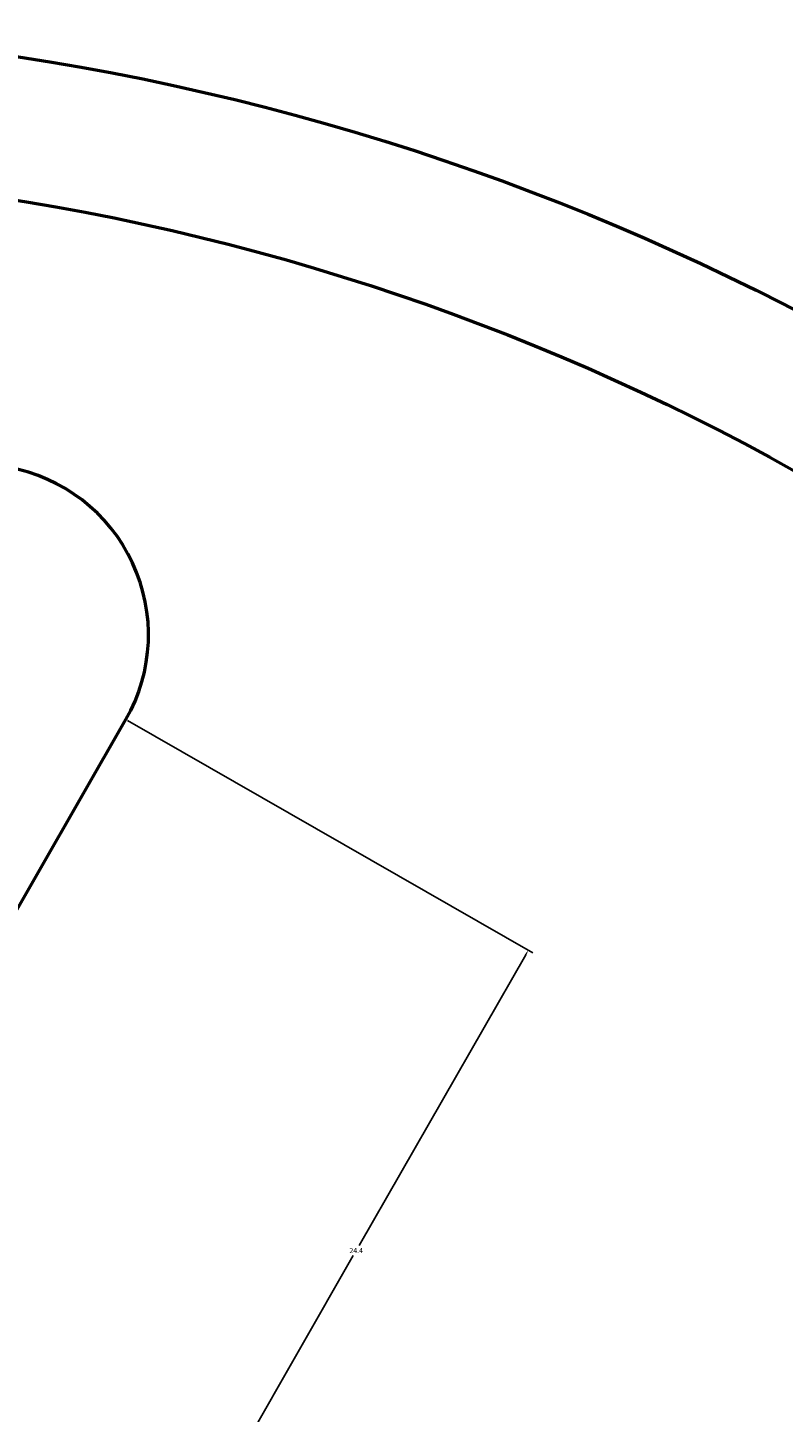
# Model space of a CAD drawing. Units: inches. Extents: x -99 to 284, y -92 to 134.
# Tile 10 of 16: x 46 to 72, y 55 to 104. Entities that reach past the tile are written whole.
import ezdxf

# ---------------------------------------------------------------- set-up
doc = ezdxf.new("R2010")
doc.units = ezdxf.units.IN
doc.header["$MEASUREMENT"] = 0
doc.layers.add('M-DIMS', color=2, linetype='Continuous', lineweight=18)
doc.layers.add('M-OUTL', color=7, linetype='Continuous', lineweight=50)
doc.styles.get("Standard").update_dxf_attribs({"font": 'arial.ttf'})
doc.dimstyles.get("Standard").update_dxf_attribs({"dimtxt": 0.18, "dimasz": 0.18, "dimexe": 0.18, "dimexo": 0.0625, "dimgap": 0.09, "dimtad": 0, "dimtih": 1, "dimtoh": 1, "dimdec": 4, "dimzin": 0, "dimdsep": 46, "dimtxsty": 'Standard', "dimcen": 0.09, "dimadec": 0, "dimazin": 0, "dimtfac": 1, "dimtdec": 4, "dimtofl": 0, "dimtmove": 0, "dimatfit": 3, "dimfxl": 1, "dimtolj": 1, "dimtzin": 0, "dimarcsym": 0})

# ---------------------------------------------------------------- blocks, each defined once
blk = doc.blocks.new('*U1')
for p, q in [((-5.205, -13.52), (-17.34, 7.646)), ((5.205, -13.52), (17.34, 7.646))]:
    blk.add_line(p, q)
for centre, start, end in [((-12.135, 10.63), 100.177, 209.8264), ((12.135, 10.63), 330.1736, 79.823), ((0, -10.536), 209.8264, 330.1736)]:
    blk.add_arc(centre, 6, start, end)
blk = doc.blocks.new('*U2')
at = {"layer": 'M-OUTL', "color": 0, "linetype": 'ByBlock', "lineweight": -2, "transparency": 16777216}
blk.add_blockref('*U1', (31.976, 71.823), dxfattribs=at)
blk = doc.blocks.new('*D14')
at = {"layer": 'Defpoints', "color": 0, "transparency": 16777216}
for p in [(49.317, 79.47), (37.182, 58.303), (51.366, 50.171)]:
    blk.add_point(p, dxfattribs=at)
at = {"layer": 'M-DIMS', "color": 0, "lineweight": -2, "transparency": 16777216}
for p, q in [((49.371, 79.439), (63.657, 71.248)), ((63.412, 71.181), (57.537, 60.935)), ((51.455, 50.327), (57.33, 60.574)), ((37.236, 58.272), (51.522, 50.082))]:
    blk.add_line(p, q, dxfattribs=at)
at = {"layer": 'M-DIMS', "color": 0, "transparency": 16777216}
for points in [[(63.385, 71.196), (63.438, 71.167), (63.501, 71.338)], [(51.429, 50.342), (51.481, 50.312), (51.366, 50.171)]]:
    blk.add_solid(points, dxfattribs=at)
at = {"layer": 'M-DIMS', "color": 0, "transparency": 16777216, "insert": (57.433, 60.754), "char_height": 0.18, "attachment_point": 5}
blk.add_mtext('\\A1;24.4', dxfattribs=at)
blk = doc.blocks.new('*D20')
at = {"layer": 'Defpoints', "color": 0, "transparency": 16777216}
for p in [(-35.23, 65.245), (99.183, -35.537)]:
    blk.add_point(p, dxfattribs=at)
at = {"layer": 'M-DIMS', "color": 0, "lineweight": -2, "transparency": 16777216}
for p, q in [((31.886, 14.854), (32.066, 14.854)), ((31.976, 14.764), (31.976, 14.944)), ((139.507, -65.772), (99.327, -35.645)), ((139.687, -65.772), (139.507, -65.772))]:
    blk.add_line(p, q, dxfattribs=at)
at = {"layer": 'M-DIMS', "color": 0, "transparency": 16777216}
blk.add_solid([(99.345, -35.621), (99.309, -35.669), (99.183, -35.537)], dxfattribs=at)
at = {"layer": 'M-DIMS', "color": 0, "transparency": 16777216, "insert": (140.074, -65.772), "char_height": 0.18, "attachment_point": 5}
blk.add_mtext('\\A1;∅168', dxfattribs=at)

msp = doc.modelspace()

# ---------------------------------------------------------------- linework, layer by layer
at = {"layer": 'M-OUTL'}
for radius in [89, 84]:
    msp.add_circle((31.9765, 14.8539), radius, dxfattribs=at)

# ---------------------------------------------------------------- block references
msp.add_blockref('*U2', (0, 0), dxfattribs=at)

# ---------------------------------------------------------------- dimensions: what is measured, and where the dimension line sits
at = {"layer": 'M-DIMS'}
dim = msp.add_linear_dim(base=(51.3659, 50.1711), p1=(49.3168, 79.4697), p2=(37.1817, 58.3032), angle=240.17365, dimstyle='Standard', override={"dimdec": 1, "dimlfac": 1, "dimrnd": 0, "dimzin": 0, "dimdsep": 46, "dimlunit": 2}, dxfattribs=at)
dim.commit()
dim.dimension.update_dxf_attribs({"geometry": '*D14', "text_midpoint": (57.4335, 60.7544)})
dim = msp.add_diameter_dim_2p(p1=(-35.2301, 65.2451), p2=(99.1831, -35.5373), dimstyle='Standard', override={"dimdec": 0, "dimlfac": 1, "dimrnd": 0, "dimzin": 0, "dimdsep": 46, "dimlunit": 2}, dxfattribs=at)
dim.commit()
dim.dimension.update_dxf_attribs({"geometry": '*D20', "text_midpoint": (140.074, -65.772), "dimtype": 163})

doc.saveas('drawing.dxf')
